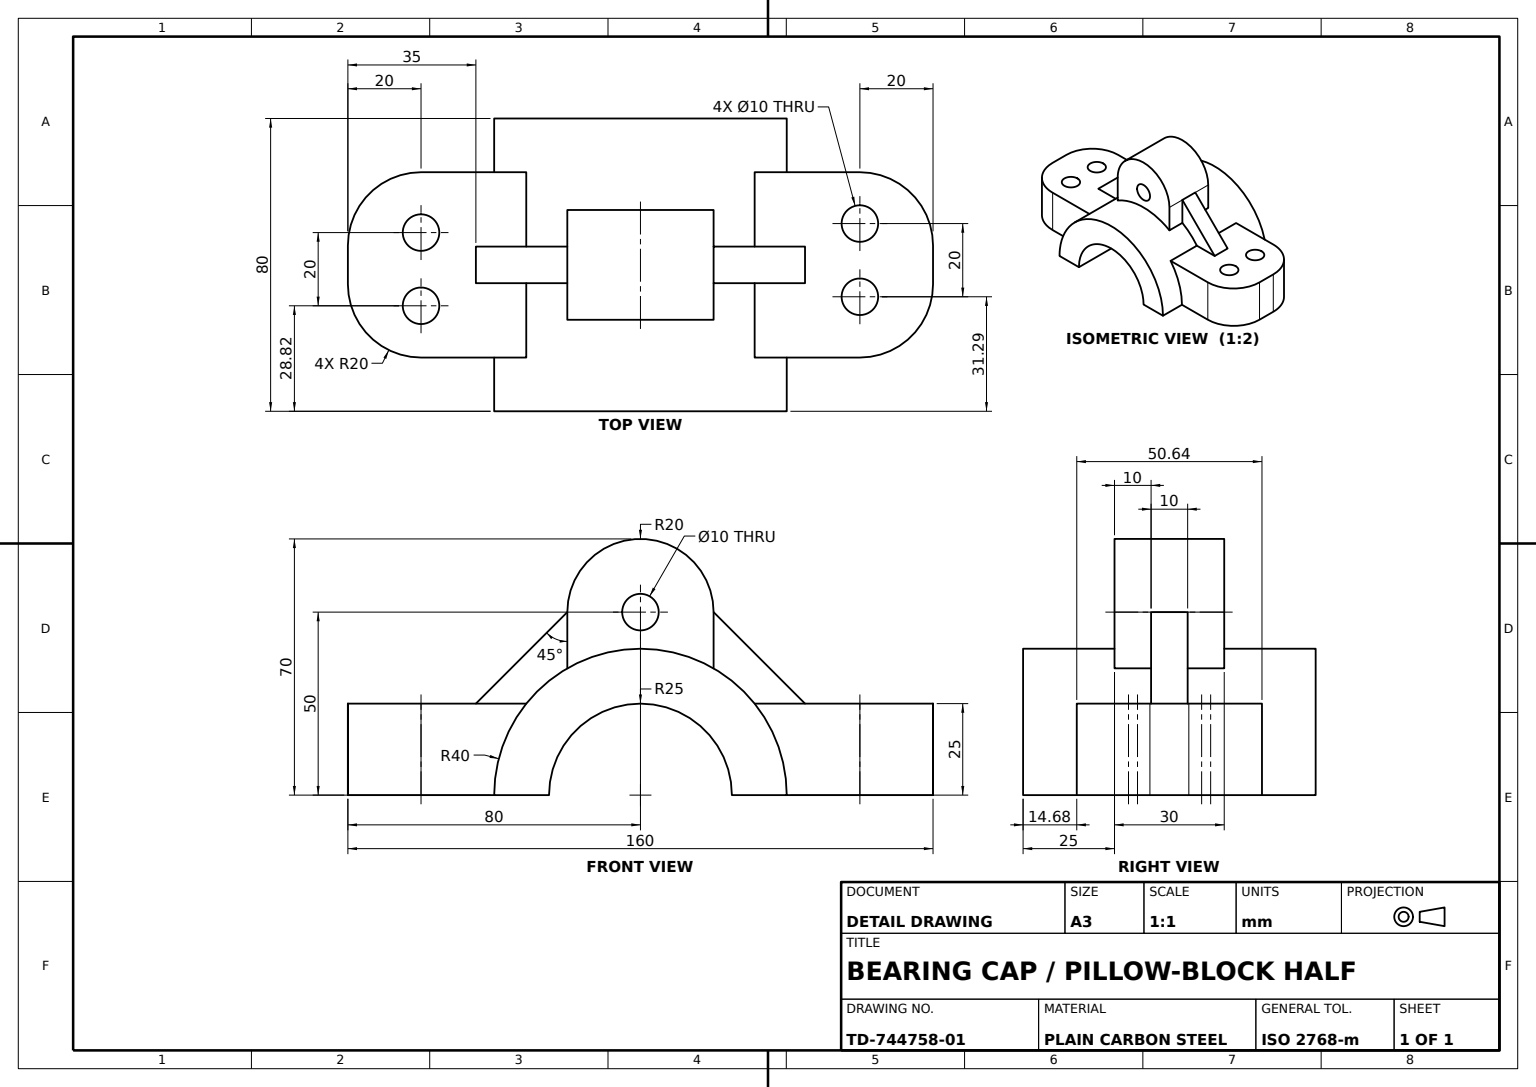
SolidWorks part; units mm, degrees
material "Plain Carbon Steel"
ref_plane "Front Plane" through (0, 0, 0) normal (0, 0, 1) x (1, 0, 0)
ref_plane "Top Plane" through (0, 0, 0) normal (0, 1, 0) x (1, 0, 0)
ref_plane "Right Plane" through (0, 0, 0) normal (1, 0, 0) x (0, 0, -1)
sketch "Housing Block Sketch" plane through (0, 0, 0) normal (0, 0, 1) x (1, 0, 0)
  line L0 (-40, 0) -> (-25, 0)
  line L1 (25, 0) -> (40, 0)
  arc A0 (40, 0) -> (-40, 0) centre (0, 0) ccw
  arc A1 (25, 0) -> (-25, 0) centre (0, 0) ccw
  dimension "D1" = 80
  dimension "D2" = 50
extrude "Housing Block" add sketch "Housing Block Sketch" against normal mid plane 80
sketch "Top Lug Sketch" plane through (0, 0, 0) normal (0, 0, 1) x (1, 0, 0)
  line L4 (-20, 50) -> (-20, 34.0024)
  line L5 (20, 50) -> (20, 34.641)
  line L6 (20, 34.641) -> (-20, 34.0024)
  arc A1 (40, 0) -> (-40, 0) centre (0, 0) ccw construction
  circle A4 centre (0, 50) radius 5
  arc A5 (20, 50) -> (-20, 50) centre (0, 50) ccw
  dimension "D1" = 50
  dimension "D2" = 20
  dimension "D3" = 10
  dimension "D4" = 15.9976
extrude "Top Lug" add sketch "Top Lug Sketch" along normal mid plane 30
sketch "Base Flange Sketch" plane through (0, 0, 0) normal (0, 1, 0) x (1, 0, 0)
  line L0 (0, -40) -> (0, 0) construction
  line L1 (-25, -40) -> (25, -40) construction
  line L2 (0, 0) -> (-71.4114, 0) construction
  line L3 (80, 25.3212) -> (80, -25.3212)
  line L4 (10, -25.3212) -> (80, -25.3212)
  line L5 (-10, 25.3212) -> (-80, 25.3212)
  line L6 (-10, 25.3212) -> (-10, -25.3212)
  line L7 (-10, -25.3212) -> (-80, -25.3212)
  line L8 (-80, 25.3212) -> (-80, -25.3212)
  line L9 (10, 25.3212) -> (10, -25.3212)
  line L10 (10, 25.3212) -> (80, 25.3212)
  dimension "D1" = 80
  dimension "D2" = 50.6424
  dimension "D3" = 10
extrude "Base Flange" add sketch "Base Flange Sketch" along normal blind 25
sketch "Bearing Seat Sketch" plane through (0, 0, 25.3212) normal (0, 0, 1) x (1, 0, 0)
  line L0 (-10, 22.9129) -> (-10, 0) construction
  line L1 (-10, 22.9129) -> (-10, 0)
  line L2 (-10, 0) -> (-25, 0)
  line L3 (10, 22.9129) -> (10, 0)
  line L4 (10, 0) -> (25, 0)
  arc A0 (-25, 0) -> (-10, 22.9129) centre (0, 0) cw
  arc A1 (25, 0) -> (-25, 0) centre (0, 0) ccw construction
  arc A2 (25, 0) -> (10, 22.9129) centre (0, 0) ccw
extrude "Bearing Seat Cut" cut sketch "Bearing Seat Sketch" against normal blind 80
fillet "Flange End Round R20 A" radius 20 3 edges at (80, 12.5, -25.3212) (80, 12.5, 25.3212) (-80, 12.5, 25.3212)
fillet "Flange End Round R20 B" radius 20 1 edges at (-80, 12.5, -25.3212)
sketch "Mounting Holes Set 1 Sketch" plane through (0, 25, 0) normal (0, 1, 0) x (1, 0, 0)
  line L0 (-80, 5.3212) -> (-80, -5.3212) construction
  line L1 (-31.225, 25.3212) -> (-60, 25.3212) construction
  circle A0 centre (-60, 8.8245) radius 5
  circle A1 centre (-60, -11.1755) radius 5
  dimension "D2" = 10
  dimension "D3" = 10
  dimension "D1" = 20
  dimension "D4" = 20
  dimension "D5" = 16.4967
extrude "Mounting Holes Set 1" cut sketch "Mounting Holes Set 1 Sketch" against normal blind 25
sketch "Mounting Holes Set 2 Sketch" plane through (0, 25, 0) normal (0, 1, 0) x (1, 0, 0)
  line L0 (80, -5.3212) -> (80, 5.3212) construction
  line L1 (60, 25.3212) -> (31.225, 25.3212) construction
  circle A0 centre (60, 11.2887) radius 5
  circle A1 centre (60, -8.7113) radius 5
  dimension "D2" = 10
  dimension "D3" = 10
  dimension "D1" = 20
  dimension "D4" = 20
  dimension "D5" = 14.0325
extrude "Mounting Holes Set 2" cut sketch "Mounting Holes Set 2 Sketch" against normal blind 25
sketch "Support Rib 1 Sketch" plane through (0, 0, 0) normal (0, 0, 1) x (1, 0, 0)
  line L0 (-20, 50) -> (-45, 25)
  line L1 (-60, 25) -> (-31.225, 25) construction
  dimension "D1" = 50
  dimension "D2" = 45
rib "Support Rib 1" sketch "Support Rib 1 Sketch" sketch "Support Rib 1 Sketch" thickness 10 extrusion direction parallel to sketch draft on no parameters "D1"=10
sketch "Support Rib 2 Sketch" plane through (0, 0, 0) normal (0, 0, 1) x (1, 0, 0)
  line L0 (20, 50) -> (45, 25)
  line L1 (31.225, 25) -> (60, 25) construction
  dimension "D1" = 50
  dimension "D2" = 45
rib "Support Rib 2" sketch "Support Rib 2 Sketch" sketch "Support Rib 2 Sketch" thickness 10 extrusion direction parallel to sketch draft on no parameters "D1"=10
